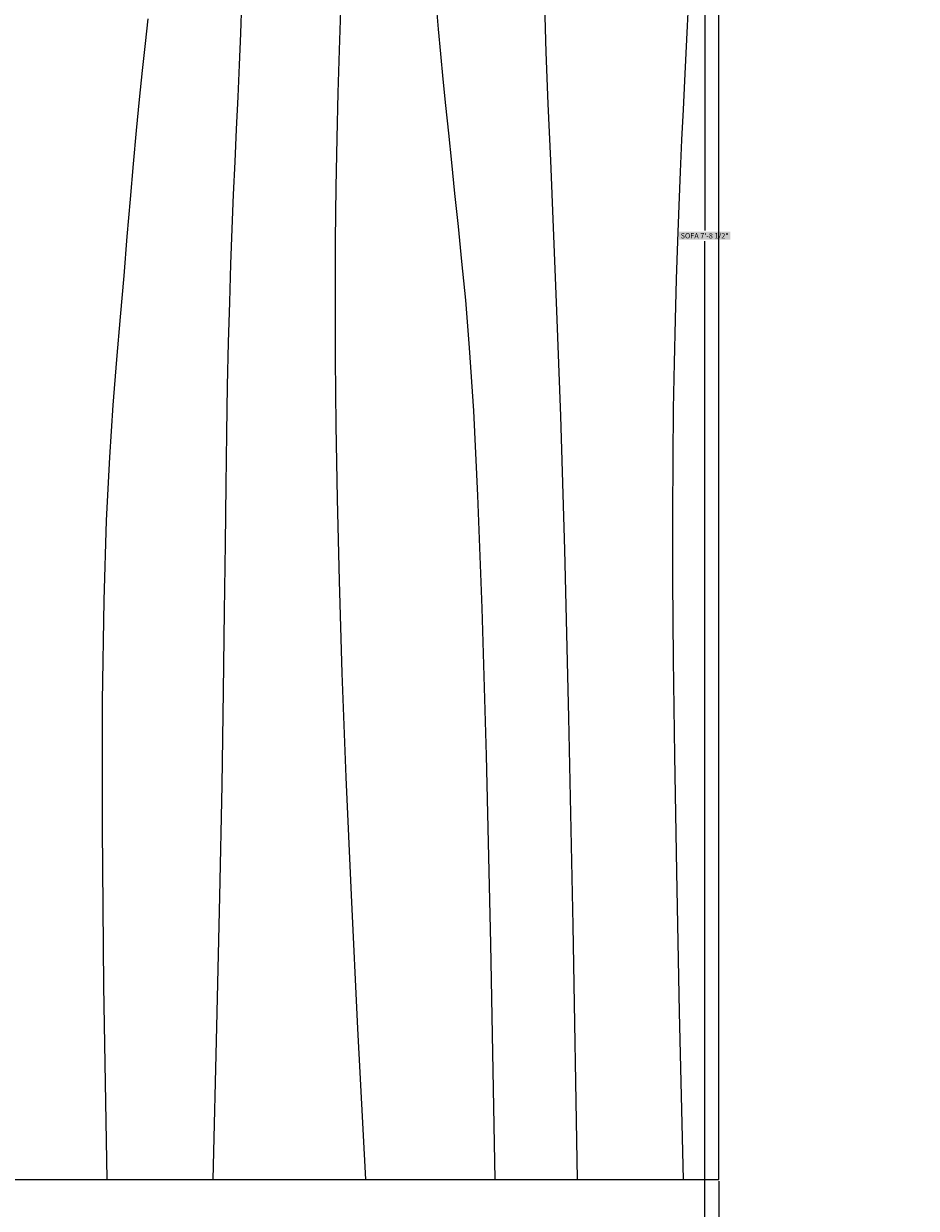
# Model space of a CAD drawing. Units: inches. Extents: x -301 to 715, y -607 to 364.
# Tile 107 of 141: x 46 to 77, y 67 to 107. Entities that reach past the tile are written whole.
import ezdxf

# ---------------------------------------------------------------- set-up
doc = ezdxf.new("R2010")
doc.units = ezdxf.units.IN
doc.header["$MEASUREMENT"] = 0
doc.layers.add('A-ANNO-DIMS', color=2, linetype='Continuous', lineweight=18)
doc.layers.add('A-FURN', color=8, linetype='Continuous', lineweight=18)
doc.styles.get("Standard").update_dxf_attribs({"font": 'arial.ttf'})
doc.dimstyles.get("Standard").update_dxf_attribs({"dimtxt": 0.18, "dimasz": 0.18, "dimexe": 0.18, "dimexo": 0.0625, "dimgap": 0.09, "dimtad": 0, "dimtih": 1, "dimtoh": 1, "dimdec": 1, "dimzin": 0, "dimdsep": 46, "dimlunit": 4, "dimtxsty": 'Standard', "dimcen": 0.09, "dimclrd": 3, "dimclre": 4, "dimclrt": 6, "dimadec": 0, "dimazin": 0, "dimtfac": 1, "dimtdec": 1, "dimtofl": 0, "dimtmove": 0, "dimatfit": 3, "dimfxl": 1, "dimtfill": 2, "dimtfillclr": 51, "dimtolj": 1, "dimtzin": 0, "dimarcsym": 0})

# ---------------------------------------------------------------- blocks, each defined once
blk = doc.blocks.new('Table - Rectangular Woodgrain 60 x 30 in.')
for p, q in [((0, 0), (0, -30)), ((0, -30), (60, -30))]:
    blk.add_line(p, q)
for points in [[(0, -9.2), (6.5759, -9.0858), (11.9385, -9.0365), (16.2527, -9.0418), (19.6833, -9.0917), (22.3952, -9.1759), (24.5531, -9.2844), (26.322, -9.4069), (27.8666, -9.5333), (29.3241, -9.6553), (30.7203, -9.7719), (32.0532, -9.8837), (33.3208, -9.9917), (34.5213, -10.0965), (35.6526, -10.199), (36.7128, -10.2999), (37.7, -10.4), (38.6129, -10.4996), (39.4531, -10.5969)], [(0, -12.8), (5.1847, -12.9322), (9.6213, -13.0323), (13.3963, -13.1059), (16.5958, -13.1583), (19.3063, -13.1952), (21.614, -13.2219), (23.6054, -13.2439), (25.3666, -13.2667), (26.9728, -13.2947), (28.4531, -13.3281), (29.8256, -13.3663), (31.1083, -13.4083), (32.3191, -13.4535), (33.476, -13.501), (34.597, -13.5501), (35.7, -13.6), (36.7984, -13.6497), (37.8875, -13.6979), (38.9578, -13.743), (40, -13.7833)], [(0, -18), (5.124, -17.7273), (9.6609, -17.5057), (13.6705, -17.3303), (17.2125, -17.1958), (20.3467, -17.0973), (23.1328, -17.0297), (25.6307, -16.9878), (27.9, -16.9667), (29.9928, -16.9617), (31.9302, -16.9703), (33.7254, -16.9907), (35.3917, -17.0208), (36.9423, -17.0588), (38.3906, -17.1026), (39.7499, -17.1503)], [(0, -22.4), (8.0098, -22.2501), (14.4094, -22.1011), (19.4168, -21.9535), (23.25, -21.8083), (26.1269, -21.6663), (28.2656, -21.5281), (29.884, -21.3947), (31.2, -21.2667), (32.3967, -21.1448), (33.5172, -21.0292), (34.5697, -20.9198), (35.5625, -20.8167), (36.5037, -20.7198), (37.4015, -20.6292), (38.2642, -20.5448), (39.1, -20.4667), (39.9164, -20.3951)], [(0, -25.2), (8.6355, -25.0504), (15.7026, -24.9031), (21.4049, -24.7606), (25.9458, -24.625), (29.529, -24.4988), (32.3578, -24.3844), (34.6359, -24.284), (36.5667, -24.2), (38.3213, -24.1341), (39.9417, -24.0854)], [(0, -28.8), (5.6867, -28.6681), (10.45, -28.5698), (14.407, -28.5012), (17.675, -28.4584), (20.3711, -28.4374), (22.6125, -28.4344), (24.5164, -28.4455), (26.2, -28.4667), (27.762, -28.4947), (29.2276, -28.5281), (30.6033, -28.5663), (31.8958, -28.6084), (33.1118, -28.6535), (34.2578, -28.7011), (35.3405, -28.7501), (36.3666, -28.8), (37.3443, -28.8497), (38.288, -28.8974), (39.2137, -28.9412), (40.1375, -28.9792)]]:
    blk.add_lwpolyline(points)
blk = doc.blocks.new('*D131')
at = {"layer": 'A-ANNO-DIMS', "color": 4, "lineweight": -2, "transparency": 16777216}
for p, q in [((39.897, 67.588), (39.897, 58.471)), ((69.897, 67.588), (69.897, 58.471))]:
    blk.add_line(p, q, dxfattribs=at)
at = {"layer": 'A-ANNO-DIMS', "color": 3, "lineweight": -2, "transparency": 16777216}
for p, q in [((40.077, 58.651), (54.566, 58.651)), ((69.717, 58.651), (55.228, 58.651))]:
    blk.add_line(p, q, dxfattribs=at)
at = {"layer": 'A-ANNO-DIMS', "color": 3, "transparency": 16777216}
for points in [[(40.077, 58.681), (40.077, 58.621), (39.897, 58.651)], [(69.717, 58.681), (69.717, 58.621), (69.897, 58.651)]]:
    blk.add_solid(points, dxfattribs=at)
at = {"layer": 'Defpoints', "color": 0, "transparency": 16777216}
for p in [(39.897, 67.651), (69.897, 67.651), (39.897, 58.651)]:
    blk.add_point(p, dxfattribs=at)
at = {"layer": 'A-ANNO-DIMS', "color": 6, "transparency": 16777216, "insert": (54.897, 58.651), "char_height": 0.18, "attachment_point": 5, "bg_fill": 1, "box_fill_scale": 1.25, "bg_fill_color": 51, "bg_fill_transparency": 0}
blk.add_mtext('\\A1;2\'-6"', dxfattribs=at)
blk = doc.blocks.new('*D132')
at = {"layer": 'A-ANNO-DIMS', "color": 4, "lineweight": -2, "transparency": 16777216}
for p, q in [((83.224, 145.954), (69.239, 145.954)), ((83.224, 53.504), (69.239, 53.504))]:
    blk.add_line(p, q, dxfattribs=at)
at = {"layer": 'A-ANNO-DIMS', "color": 3, "lineweight": -2, "transparency": 16777216}
for p, q in [((69.419, 145.774), (69.419, 99.912)), ((69.419, 53.684), (69.419, 99.546))]:
    blk.add_line(p, q, dxfattribs=at)
at = {"layer": 'A-ANNO-DIMS', "color": 3, "transparency": 16777216}
for points in [[(69.389, 145.774), (69.449, 145.774), (69.419, 145.954)], [(69.389, 53.684), (69.449, 53.684), (69.419, 53.504)]]:
    blk.add_solid(points, dxfattribs=at)
at = {"layer": 'Defpoints', "color": 0, "transparency": 16777216}
for p in [(83.287, 145.954), (69.419, 53.504), (83.287, 53.504)]:
    blk.add_point(p, dxfattribs=at)
at = {"layer": 'A-ANNO-DIMS', "color": 6, "transparency": 16777216, "insert": (69.419, 99.729), "char_height": 0.18, "attachment_point": 5, "bg_fill": 1, "box_fill_scale": 1.25, "bg_fill_color": 51, "bg_fill_transparency": 0}
blk.add_mtext('\\A1;SOFA 7\'-8 1/2"', dxfattribs=at)

msp = doc.modelspace()

# ---------------------------------------------------------------- block references
at = {"layer": 'A-FURN', "rotation": 90}
msp.add_blockref('Table - Rectangular Woodgrain 60 x 30 in.', (39.897, 67.651), dxfattribs=at)

# ---------------------------------------------------------------- dimensions: what is measured, and where the dimension line sits
at = {"layer": 'A-ANNO-DIMS'}
dim = msp.add_linear_dim(base=(69.4192, 53.5044), p1=(83.2867, 145.9543), p2=(83.2867, 53.5044), angle=270, text='SOFA <>', dimstyle='Standard', override={"dimdec": 1, "dimlfac": 1, "dimrnd": 0, "dimzin": 1, "dimdsep": 46, "dimlunit": 4, "dimfrac": 2}, dxfattribs=at)
dim.commit()
dim.dimension.update_dxf_attribs({"geometry": '*D132', "text_midpoint": (69.4192, 99.7293)})
dim = msp.add_linear_dim(base=(39.897, 58.651), p1=(69.897, 67.651), p2=(39.897, 67.651), angle=180, dimstyle='Standard', override={"dimdec": 1, "dimlfac": 1, "dimrnd": 0, "dimzin": 1, "dimdsep": 46, "dimlunit": 4, "dimfrac": 2}, dxfattribs=at)
dim.commit()
dim.dimension.update_dxf_attribs({"geometry": '*D131', "text_midpoint": (54.897, 58.651)})

doc.saveas('drawing.dxf')
